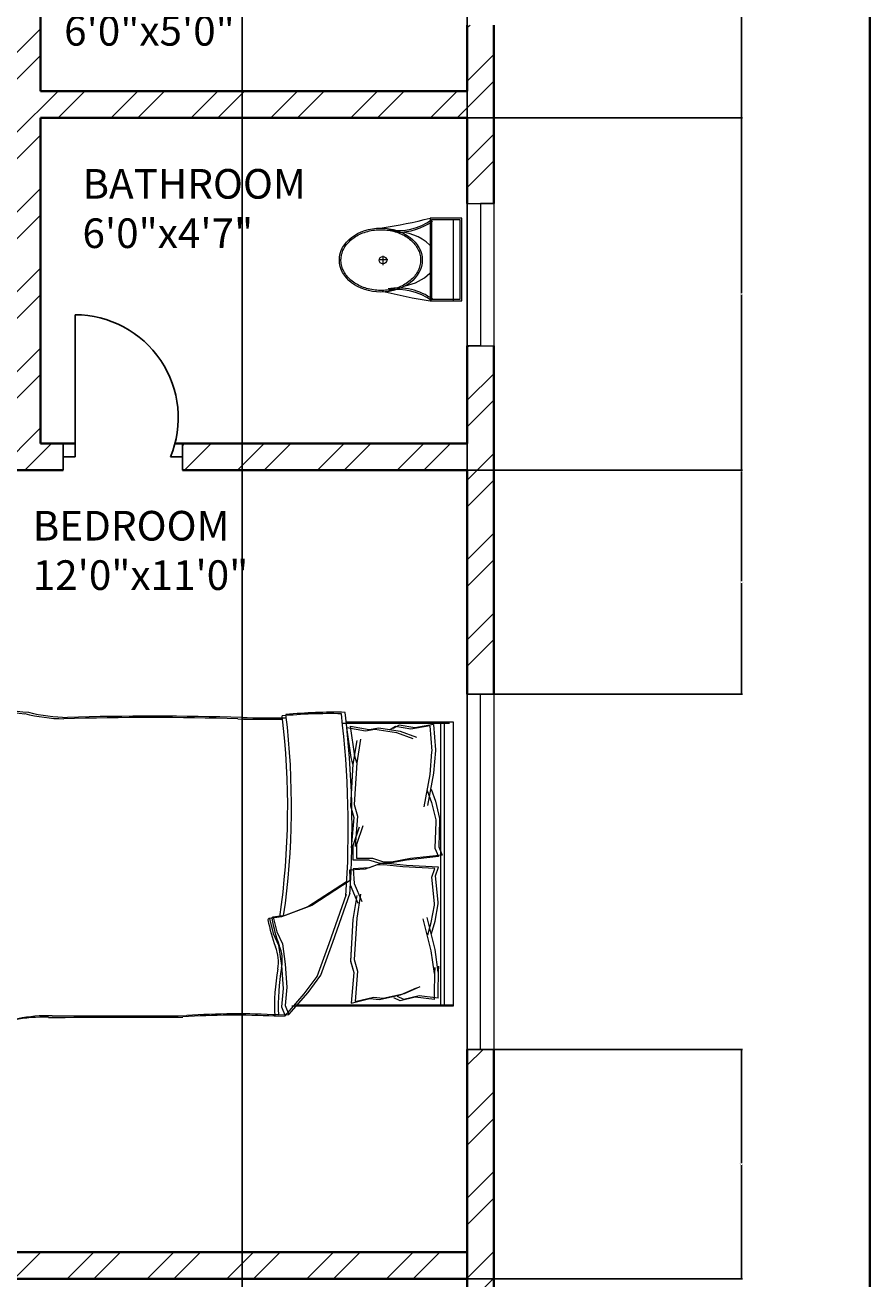
# Model space of a CAD drawing. Units: inches. Extents: x 2063 to 2617, y 1299 to 2210.
# Tile 20 of 22: x 2475 to 2617, y 1727 to 1939. Entities that reach past the tile are written whole.
import ezdxf

# ---------------------------------------------------------------- set-up
doc = ezdxf.new("R2010")
doc.units = ezdxf.units.IN
for name, color, linetype, lineweight in [('A-ANNO-DIMS', 2, 'Continuous', 18), ('A-ANNO-TTLB', 7, 'Continuous', 35), ('A-AREA-IDEN', 7, 'Continuous', 18), ('A-DOOR', 11, 'Continuous', 25), ('A-FLOR-FIXT', 8, 'Continuous', 18), ('A-FURN', 8, 'Continuous', 18), ('A-GLAZ', 123, 'Continuous', 18), ('A-WALL', 7, 'Continuous', 40)]:
    doc.layers.add(name, color=color, linetype=linetype, lineweight=lineweight)
doc.layers.add('A-WALL-PATT', color=215, linetype='Continuous', lineweight=13, true_color=0xa953a0)
doc.styles.get("Standard").update_dxf_attribs({"font": 'arial.ttf'})
doc.dimstyles.get("Standard").update_dxf_attribs({"dimtxt": 0.18, "dimasz": 0.18, "dimexe": 0.18, "dimexo": 0.0625, "dimgap": 0.09, "dimtad": 0, "dimtih": 1, "dimtoh": 1, "dimdec": 4, "dimzin": 0, "dimdsep": 46, "dimtxsty": 'Standard', "dimcen": 0.09, "dimadec": 0, "dimazin": 0, "dimtfac": 1, "dimtdec": 4, "dimtofl": 0, "dimtmove": 0, "dimatfit": 3, "dimfxl": 1, "dimtolj": 1, "dimtzin": 0, "dimarcsym": 0})

# ---------------------------------------------------------------- blocks, each defined once
blk = doc.blocks.new('A$C31115884')
for p, q in [((283.1, 497.7), (223.4, 497.7)), ((257.5, 466.4), (257.5, 523.2)), ((0, 200), (0, 0)), ((520, 200), (0, 200)), ((10, 190), (10, 10)), ((510, 190), (10, 190)), ((510, 10), (510, 190)), ((520, 0), (520, 200)), ((510, 54.5), (0, 54.5)), ((10, 10), (510, 10)), ((0, 0), (520, 0))]:
    blk.add_line(p, q)
blk.add_circle((255.6, 496.4), 23.6)
for centre, radius, start, end in [((2777.7, -204.6), 2807, 165.4549, 171.71327), ((3237, 905), 2807, 188.28673, 194.5451), ((-294.5, 403.3), 364.7, 324.20913, 9.34987), ((-294.5, 403.3), 374.7, 324.20913, 9.34987), ((139.5, 406.2), 293.5, 315.84364, 2.65635), ((805.8, 403.3), 374.7, 179.20365, 215.79087), ((805.8, 403.3), 364.7, 170.65013, 215.79087), ((383.6, 406.2), 293.5, 190.27735, 224.15636)]:
    blk.add_arc(centre, radius, start, end)
blk.add_ellipse((256.2, 509.9), major_axis=(0, -260.7), ratio=0.772727)
blk.add_open_spline([(256.2, 259.2), (263.1, 259.2), (270, 259.7), (287.8, 262.3), (298.7, 265.1), (319.9, 273.1), (330.2, 278.4), (350.1, 291.1), (359.7, 298.7), (377.7, 315.9), (386.2, 325.5), (401.7, 346.6), (408.8, 358.1), (421.3, 382.5), (426.8, 395.5), (435.9, 422.4), (439.5, 436.4), (444.8, 465.1), (446.5, 479.7), (447.9, 509.2), (447.6, 524), (445, 553.3), (442.7, 567.8), (436.3, 596), (432.1, 609.7), (421.9, 636), (416, 648.6), (402.5, 672.1), (395, 683), (378.6, 703), (369.8, 712.1), (351.1, 728), (341.3, 734.8), (320.9, 746.2), (310.4, 750.7), (288.9, 757.3), (278, 759.4), (256, 761), (245, 760.6), (223.1, 757.2), (212.3, 754.3), (191.1, 746.1), (180.8, 740.7), (160.9, 727.8), (151.4, 720.1), (133.5, 702.7), (125.1, 693), (109.6, 671.7), (102.6, 660.2), (90.2, 635.7), (84.9, 622.7), (76, 595.6), (72.4, 581.6), (67.2, 552.9), (65.6, 538.2), (64.4, 508.8), (64.8, 494), (67.5, 464.7), (69.9, 450.2), (76.6, 422), (80.8, 408.3), (91.1, 382.2), (97.2, 369.7), (110.8, 346.3), (118.4, 335.4), (134.8, 315.6), (143.7, 306.7), (162.4, 290.9), (172.3, 284.2), (192.8, 273), (203.3, 268.6), (224.8, 262.2), (235.8, 260.2), (249.9, 259.3), (253, 259.2), (256.2, 259.2)], degree=3, knots=[0, 0, 0, 0, 0.110105, 0.110105, 0.285049, 0.285049, 0.459994, 0.459994, 0.634938, 0.634938, 0.809882, 0.809882, 0.984827, 0.984827, 1.159771, 1.159771, 1.334715, 1.334715, 1.50966, 1.50966, 1.684604, 1.684604, 1.859549, 1.859549, 2.034493, 2.034493, 2.209437, 2.209437, 2.384382, 2.384382, 2.559326, 2.559326, 2.73427, 2.73427, 2.909215, 2.909215, 3.084159, 3.084159, 3.259103, 3.259103, 3.434048, 3.434048, 3.608992, 3.608992, 3.783936, 3.783936, 3.958881, 3.958881, 4.133825, 4.133825, 4.30877, 4.30877, 4.483714, 4.483714, 4.658658, 4.658658, 4.833603, 4.833603, 5.008547, 5.008547, 5.183491, 5.183491, 5.358436, 5.358436, 5.53338, 5.53338, 5.708324, 5.708324, 5.883269, 5.883269, 6.058213, 6.058213, 6.233158, 6.233158, 6.283185, 6.283185, 6.283185, 6.283185])
blk = doc.blocks.new('BED-DOUBLE')
for p, q in [((3.48, 63.33), (3.48, 81.44)), ((3.48, 63.33), (3.48, 81.44)), ((3.48, 81.44), (51.49, 81.44)), ((3.7, 62.69), (3.7, 80.8)), ((3.7, 62.69), (3.7, 80.8)), ((51.27, 81.44), (51.27, 54.83)), ((51.27, 81.44), (51.27, 54.83)), ((51.49, 81.44), (51.49, 80.8)), ((51.49, 80.8), (51.49, 54.19)), ((51.49, 80.8), (51.49, 54.19)), ((3.48, 79.91), (51.27, 79.91)), ((3.48, 79.91), (51.27, 79.91)), ((3.7, 79.27), (51.49, 79.27)), ((3.7, 79.27), (51.49, 79.27)), ((3.9, 78.11), (8.18, 78.43)), ((3.9, 78.11), (8.18, 78.43)), ((8.18, 78.43), (8.29, 78.42)), ((8.18, 78.43), (8.29, 78.42)), ((8.29, 78.42), (12.11, 78.13)), ((8.29, 78.42), (12.11, 78.13)), ((14.86, 77.69), (16.88, 78.42)), ((14.86, 77.69), (16.88, 78.42)), ((16.88, 78.42), (19.77, 79.14)), ((16.88, 78.42), (19.77, 79.14)), ((17.11, 77.78), (20, 78.5)), ((17.11, 77.78), (20, 78.5)), ((19.77, 79.14), (20.09, 79.14)), ((19.77, 79.14), (20.09, 79.14)), ((20, 78.5), (20.32, 78.5)), ((20, 78.5), (20.32, 78.5)), ((20.09, 79.14), (24.54, 79)), ((20.09, 79.14), (24.54, 79)), ((20.32, 78.5), (24.77, 78.36)), ((20.32, 78.5), (24.77, 78.36)), ((24.54, 79), (25.98, 79.57)), ((24.54, 79), (25.98, 79.57)), ((24.77, 78.36), (26.21, 78.93)), ((24.77, 78.36), (26.21, 78.93)), ((25.98, 79.57), (26.56, 74.22)), ((25.98, 79.57), (26.56, 74.22)), ((26.21, 78.93), (26.79, 73.58)), ((26.21, 78.93), (26.79, 73.58)), ((27.98, 78.95), (27.73, 73.58)), ((27.98, 78.95), (27.73, 73.58)), ((29.46, 78.46), (27.98, 78.95)), ((29.46, 78.46), (27.98, 78.95)), ((33.88, 78.89), (29.46, 78.46)), ((33.88, 78.89), (29.46, 78.46)), ((34.21, 78.91), (33.88, 78.89)), ((34.2, 78.91), (33.88, 78.89)), ((37.14, 78.37), (34.2, 78.91)), ((37.14, 78.37), (34.21, 78.91)), ((41.91, 78.37), (36.5, 77.02)), ((41.91, 78.37), (36.5, 77.02)), ((39.2, 77.77), (37.14, 78.37)), ((39.2, 77.77), (37.14, 78.37)), ((45.71, 78.9), (41.91, 78.37)), ((45.71, 78.9), (41.91, 78.37)), ((50.11, 78.89), (44.71, 78.98)), ((44.71, 78.98), (45.71, 78.9)), ((50.11, 78.89), (44.71, 78.98)), ((44.71, 78.98), (45.71, 78.9)), ((50.34, 78.25), (44.94, 78.34)), ((44.94, 78.34), (45.94, 78.26)), ((50.34, 78.25), (44.94, 78.34)), ((44.94, 78.34), (45.94, 78.26)), ((50.11, 78.89), (49.73, 75.68)), ((50.11, 78.89), (49.73, 75.68)), ((3.89, 78.13), (4.47, 74.95)), ((3.9, 78.13), (4.47, 74.95)), ((4.12, 77.49), (4.7, 74.31)), ((4.12, 77.49), (4.7, 74.31)), ((4.13, 77.47), (8.41, 77.8)), ((4.13, 77.47), (8.41, 77.8)), ((8.41, 77.8), (8.51, 77.78)), ((8.41, 77.8), (8.51, 77.78)), ((8.51, 77.78), (12.34, 77.49)), ((8.51, 77.78), (12.34, 77.49)), ((12.11, 78.13), (17.6, 77.12)), ((12.11, 78.13), (17.6, 77.12)), ((12.34, 77.49), (17.83, 76.48)), ((12.34, 77.49), (17.83, 76.48)), ((15.08, 77.05), (17.11, 77.78)), ((15.08, 77.05), (17.11, 77.78)), ((28.21, 78.31), (27.96, 72.94)), ((28.21, 78.31), (27.96, 72.94)), ((29.68, 77.83), (28.21, 78.31)), ((29.68, 77.83), (28.21, 78.31)), ((34.11, 78.25), (29.68, 77.83)), ((34.11, 78.25), (29.68, 77.83)), ((34.43, 78.27), (34.11, 78.25)), ((34.43, 78.27), (34.11, 78.25)), ((37.36, 77.73), (34.43, 78.27)), ((37.36, 77.73), (34.43, 78.27)), ((42.14, 77.73), (36.72, 76.38)), ((42.14, 77.73), (36.72, 76.38)), ((39.43, 77.13), (37.36, 77.73)), ((39.43, 77.13), (37.36, 77.73)), ((45.94, 78.26), (42.14, 77.73)), ((45.94, 78.26), (42.14, 77.73)), ((50.34, 78.25), (49.96, 75.04)), ((50.34, 78.25), (49.96, 75.04)), ((4.47, 74.95), (4.04, 72.34)), ((4.47, 74.95), (4.04, 72.34)), ((4.7, 74.31), (4.27, 71.7)), ((4.7, 74.31), (4.27, 71.7)), ((5.05, 72.49), (6.06, 75.24)), ((5.05, 72.49), (6.06, 75.24)), ((5.28, 71.85), (6.29, 74.6)), ((5.28, 71.85), (6.29, 74.6)), ((26.56, 74.22), (27.14, 71.04)), ((26.56, 74.22), (27.14, 71.04)), ((49.31, 73.19), (48.13, 75.87)), ((49.31, 73.19), (48.13, 75.87)), ((49.54, 72.55), (48.36, 75.23)), ((49.54, 72.55), (48.36, 75.23)), ((49.73, 75.68), (50.33, 73.11)), ((49.73, 75.68), (50.33, 73.11)), ((49.96, 75.04), (50.56, 72.47)), ((49.96, 75.04), (50.56, 72.47)), ((4.04, 72.34), (4.62, 71.33)), ((4.04, 72.34), (4.62, 71.33)), ((4.47, 68.87), (5.05, 72.49)), ((4.47, 68.87), (5.05, 72.49)), ((26.79, 73.58), (27.37, 70.4)), ((26.79, 73.58), (27.37, 70.4)), ((27.73, 73.58), (27.36, 70.37)), ((27.73, 73.58), (27.36, 70.37)), ((27.96, 72.94), (27.58, 69.73)), ((27.96, 72.94), (27.58, 69.73)), ((50.11, 69.61), (49.31, 73.19)), ((50.11, 69.61), (49.31, 73.19)), ((50.34, 68.98), (49.54, 72.55)), ((50.34, 68.98), (49.54, 72.55)), ((50.33, 73.11), (49.81, 72.06)), ((50.33, 73.11), (49.82, 72.06)), ((50.56, 72.47), (50.04, 71.42)), ((50.56, 72.47), (50.04, 71.42)), ((4.27, 71.7), (4.85, 70.69)), ((4.27, 71.7), (4.85, 70.69)), ((4.7, 68.23), (5.28, 71.85)), ((4.7, 68.23), (5.28, 71.85)), ((27.14, 71.04), (27.14, 69.74)), ((27.14, 71.04), (27.14, 69.74)), ((27.36, 70.37), (27.44, 69.07)), ((27.36, 70.37), (27.44, 69.07)), ((27.37, 70.4), (27.37, 69.1)), ((27.37, 70.4), (27.37, 69.1)), ((4.76, 67.28), (4.47, 68.87)), ((4.76, 67.28), (4.47, 68.87)), ((4.99, 66.64), (4.7, 68.23)), ((4.99, 66.64), (4.7, 68.23)), ((27.14, 69.74), (26.56, 67.86)), ((27.14, 69.74), (26.56, 67.86)), ((26.56, 67.86), (26.56, 65.18)), ((26.56, 67.86), (26.56, 65.18)), ((27.37, 69.1), (26.79, 67.22)), ((27.37, 69.1), (26.79, 67.22)), ((27.44, 69.07), (28.13, 67.23)), ((27.44, 69.07), (28.13, 67.23)), ((27.58, 69.73), (27.66, 68.43)), ((27.58, 69.73), (27.66, 68.43)), ((27.66, 68.43), (28.36, 66.59)), ((27.66, 68.43), (28.36, 66.59)), ((49.92, 68.01), (50.11, 69.61)), ((49.92, 68.01), (50.11, 69.61)), ((50.7, 64.87), (49.92, 68.01)), ((50.7, 64.87), (49.92, 68.01)), ((50.15, 67.37), (50.34, 68.98)), ((50.15, 67.37), (50.34, 68.98)), ((4.18, 64.1), (4.76, 67.28)), ((4.18, 64.1), (4.76, 67.28)), ((4.41, 63.46), (4.99, 66.64)), ((4.41, 63.46), (4.99, 66.64)), ((6.38, 65.82), (10.41, 65.15)), ((6.38, 65.82), (10.41, 65.15)), ((24.1, 65.18), (20.96, 66.27)), ((24.1, 65.18), (20.96, 66.27)), ((24.33, 64.54), (21.19, 65.63)), ((24.33, 64.54), (21.19, 65.63)), ((26.79, 67.22), (26.79, 64.54)), ((26.79, 67.22), (26.79, 64.54)), ((28.13, 67.23), (28.3, 64.55)), ((28.13, 67.23), (28.3, 64.55)), ((28.36, 66.59), (28.53, 63.91)), ((28.36, 66.59), (28.53, 63.91)), ((30.75, 64.7), (33.82, 65.99)), ((30.75, 64.7), (33.82, 65.99)), ((32.56, 65.82), (36.6, 65.15)), ((32.56, 65.82), (36.6, 65.15)), ((50.93, 64.23), (50.15, 67.37)), ((50.93, 64.23), (50.15, 67.37)), ((9.28, 64.83), (4.18, 64.1)), ((9.28, 64.83), (4.18, 64.1)), ((9.51, 64.19), (4.41, 63.46)), ((9.51, 64.19), (4.41, 63.46)), ((6.61, 65.18), (10.64, 64.51)), ((6.61, 65.18), (10.64, 64.51)), ((10.41, 65.15), (9.28, 64.83)), ((10.41, 65.15), (9.28, 64.83)), ((10.64, 64.51), (9.51, 64.19)), ((10.64, 64.51), (9.51, 64.19)), ((10.41, 65.15), (17.42, 64.72)), ((10.41, 65.15), (17.42, 64.72)), ((10.64, 64.51), (17.65, 64.08)), ((10.64, 64.51), (17.65, 64.08)), ((17.42, 64.72), (19.38, 65.27)), ((17.42, 64.72), (19.38, 65.27)), ((17.65, 64.08), (19.61, 64.64)), ((17.65, 64.08), (19.61, 64.64)), ((19.38, 65.27), (24.52, 64.87)), ((19.38, 65.27), (24.52, 64.87)), ((19.61, 64.64), (24.74, 64.23)), ((19.61, 64.64), (24.74, 64.23)), ((26.56, 65.18), (24.1, 65.18)), ((26.56, 65.18), (24.1, 65.18)), ((26.79, 64.54), (24.33, 64.54)), ((26.79, 64.54), (24.33, 64.54)), ((28.3, 64.55), (30.75, 64.7)), ((28.3, 64.55), (30.75, 64.7)), ((28.53, 63.91), (30.98, 64.06)), ((28.53, 63.91), (30.98, 64.06)), ((30.26, 64.06), (34.45, 57.57)), ((30.26, 64.06), (34.45, 57.57)), ((30.98, 64.06), (34.05, 65.35)), ((30.98, 64.06), (34.05, 65.35)), ((40.64, 61.13), (32.31, 64.06)), ((40.64, 61.13), (32.31, 64.06)), ((32.79, 65.18), (36.83, 64.51)), ((32.79, 65.18), (36.82, 64.51)), ((36.6, 65.15), (43.61, 64.72)), ((36.6, 65.15), (43.61, 64.72)), ((36.82, 64.51), (43.83, 64.08)), ((36.83, 64.51), (43.84, 64.08)), ((43.61, 64.72), (45.57, 65.27)), ((43.61, 64.72), (45.57, 65.27)), ((43.83, 64.08), (45.8, 64.64)), ((43.84, 64.08), (45.8, 64.64)), ((45.57, 65.27), (50.7, 64.87)), ((45.57, 65.27), (50.7, 64.87)), ((45.8, 64.64), (50.93, 64.23)), ((45.8, 64.64), (50.93, 64.23)), ((30.49, 63.42), (34.68, 56.93)), ((30.49, 63.42), (34.68, 56.93)), ((40.87, 60.49), (32.53, 63.42)), ((40.87, 60.49), (32.54, 63.42)), ((46.22, 59.11), (40.64, 61.13)), ((46.22, 59.11), (40.64, 61.13)), ((46.45, 58.48), (40.87, 60.49)), ((46.45, 58.48), (40.87, 60.49)), ((34.45, 57.57), (36.15, 53.08)), ((34.45, 57.57), (36.15, 53.08)), ((49.16, 56.95), (46.22, 59.11)), ((49.16, 56.95), (46.22, 59.11)), ((49.39, 56.31), (46.45, 58.48)), ((49.39, 56.31), (46.45, 58.48)), ((34.68, 56.93), (36.38, 52.44)), ((34.68, 56.93), (36.38, 52.44)), ((52.87, 53.7), (49.16, 56.95)), ((52.87, 53.7), (49.16, 56.95)), ((53.1, 53.06), (49.39, 56.31)), ((53.1, 53.06), (49.39, 56.31)), ((36.15, 53.08), (36.46, 51.07)), ((36.15, 53.08), (36.46, 51.07)), ((40.95, 52.61), (44.36, 53.08)), ((40.95, 52.61), (44.36, 53.08)), ((44.36, 53.08), (48.23, 53.39)), ((44.36, 53.08), (48.23, 53.39)), ((48.23, 53.39), (51.33, 53.08)), ((48.23, 53.39), (51.33, 53.08)), ((51.33, 53.08), (52.87, 53.7)), ((51.33, 53.08), (52.87, 53.7)), ((51.56, 52.44), (53.1, 53.06)), ((51.56, 52.44), (53.1, 53.06)), ((52.95, 51.95), (52.87, 53.7, 3.87)), ((52.95, 51.95), (52.87, 53.7, 3.87)), ((53.18, 51.31), (53.1, 53.06, 3.87)), ((53.18, 51.31), (53.1, 53.06, 3.87)), ((36.38, 52.44), (36.69, 50.43)), ((36.38, 52.44), (36.69, 50.43)), ((36.46, 51.07), (38.94, 51.69)), ((36.46, 51.07), (38.94, 51.69)), ((36.69, 50.43), (39.17, 51.05)), ((36.69, 50.43), (39.17, 51.05)), ((38.94, 51.69), (40.95, 52.61)), ((38.94, 51.69), (40.95, 52.61)), ((39.17, 51.05), (41.18, 51.97)), ((39.17, 51.05), (41.18, 51.97)), ((41.18, 51.97), (44.59, 52.44)), ((41.18, 51.97), (44.59, 52.44)), ((44.59, 52.44), (48.46, 52.75)), ((44.59, 52.44), (48.46, 52.75)), ((48.46, 52.75), (51.56, 52.44)), ((48.46, 52.75), (51.56, 52.44)), ((15.06, 2.2), (39.68, 2.2)), ((15.06, 2.2), (39.68, 2.2)), ((15.29, 1.56), (39.91, 1.56)), ((15.29, 1.56), (39.91, 1.56))]:
    blk.add_line(p, q)
for centre, radius, start, end in [((21.36, -100.61), 164.97, 86.0865, 96.7821), ((21.36, -100.61), 164.97, 86.0865, 96.7821), ((21.59, -101.25), 164.97, 86.0865, 96.7821), ((21.59, -101.25), 164.97, 86.0865, 96.7821), ((85.16, 61.35), 83.31, 178.7218, 185.604), ((85.16, 61.35), 83.31, 178.7218, 185.604), ((85.39, 60.71), 83.31, 178.7218, 185.604), ((85.39, 60.71), 83.31, 178.7218, 185.604), ((17.76, -74.87), 129.02, 81.7845, 96.9006), ((17.76, -74.87), 129.02, 81.7845, 96.9006), ((17.98, -75.51), 129.02, 81.7845, 96.9006), ((17.98, -75.51), 129.02, 81.7845, 96.9006), ((-167.31, 50.27), 170.11, 358.4762, 1.0082), ((-167.31, 50.27), 170.11, 358.4762, 1.0082), ((-167.08, 49.63), 170.11, 358.4762, 1.0082), ((-167.08, 49.63), 170.11, 358.4762, 1.0082), ((36.64, 51), 0.185, 160.2464, 271.1377), ((36.64, 51), 0.185, 160.2464, 271.1377), ((31.15, 79.96), 29.65, 280.6617, 289.8806), ((31.15, 79.96), 29.65, 280.6617, 289.8806), ((31.38, 79.32), 29.65, 280.6617, 289.8806), ((31.38, 79.32), 29.65, 280.6617, 289.8806), ((43.74, 46.38), 6.22, 78.6608, 113.7384), ((43.74, 46.38), 6.22, 78.6608, 113.7384), ((43.97, 45.74), 6.22, 78.6608, 113.7384), ((43.97, 45.74), 6.22, 78.6608, 113.7384), ((51.33, 88.1), 36.18, 259.8763, 272.5657), ((51.33, 88.1), 36.18, 259.8763, 272.5657), ((51.56, 87.46), 36.18, 259.8763, 272.5657), ((51.56, 87.46), 36.18, 259.8763, 272.5657), ((182.27, 45.13), 129.5, 176.9791, 183.8365), ((182.27, 45.13), 129.5, 176.9791, 183.8365), ((182.49, 44.49), 129.5, 176.9791, 183.8365), ((182.49, 44.49), 129.5, 176.9791, 183.8365), ((36.87, 50.36), 0.185, 160.2464, 271.1377), ((36.86, 50.36), 0.185, 160.2464, 271.1377), ((484.82, 30.83), 482.31, 178.2277, 181.7185), ((484.82, 30.83), 482.31, 178.2277, 181.7185), ((485.05, 30.19), 482.31, 178.2277, 181.7185), ((485.05, 30.19), 482.31, 178.2277, 181.7185), ((-4508.74, 13.62), 4561.86, 0.00217, 0.28689), ((-4508.74, 13.62), 4561.86, 0.00217, 0.28689), ((-4508.51, 12.98), 4561.86, 0.00217, 0.28689), ((-4508.51, 12.98), 4561.86, 0.00217, 0.28689), ((-26.9, 16.93), 29.63, 346.0648, 358.9113), ((-26.9, 16.93), 29.63, 346.0648, 358.9113), ((-26.67, 16.29), 29.63, 346.0648, 358.9113), ((-26.67, 16.29), 29.63, 346.0648, 358.9113), ((76.16, 12.78), 23.07, 177.4714, 206.4681), ((76.16, 12.78), 23.07, 177.4714, 206.4681), ((76.39, 12.14), 23.07, 177.4714, 206.4681), ((76.39, 12.14), 23.07, 177.4714, 206.4681), ((-21.66, 11.17), 23.56, 337.9751, 356.652), ((-21.66, 11.17), 23.56, 337.9751, 356.652), ((-21.43, 10.53), 23.56, 337.9751, 356.652), ((-21.43, 10.53), 23.56, 337.9751, 356.652), ((1.09, 1.73), 1.09, 146.1736, 293.4781), ((1.09, 1.73), 1.09, 146.1736, 293.4781), ((21.43, -119.39), 121.76, 92.9958, 99.4091), ((21.43, -119.39), 121.76, 92.9958, 99.4091), ((-17.22, 105.16), 106.46, 283.3832, 287.7053), ((-17.22, 105.16), 106.46, 283.3832, 287.7053), ((-16.99, 104.52), 106.46, 283.3832, 287.7053), ((-16.99, 104.52), 106.46, 283.3832, 287.7053), ((41.15, -130.83), 133.04, 84.4998, 90.6351), ((41.15, -130.83), 133.04, 84.4998, 90.6351), ((54.41, 2.57), 1.1, 242.6588, 356.02), ((54.41, 2.57), 1.1, 242.6588, 356.02), ((1.32, 1.09), 1.09, 146.1736, 293.4781), ((1.32, 1.09), 1.09, 146.1736, 293.4781), ((21.66, -120.03), 121.76, 92.9958, 99.4091), ((21.66, -120.03), 121.76, 92.9958, 99.4091), ((41.38, -131.47), 133.04, 84.4998, 90.6351), ((41.38, -131.47), 133.04, 84.4998, 90.6351), ((54.64, 1.93), 1.1, 242.6588, 356.02), ((54.64, 1.93), 1.1, 242.6588, 356.02)]:
    blk.add_arc(centre, radius, start, end)
blk = doc.blocks.new('WIN-24IN')
for p, q in [((0, 24), (4.5, 24)), ((0, 24), (0, 0)), ((4.5, 24), (2.25, 24)), ((2.25, 24), (2.25, 0)), ((4.5, 24), (4.5, 0)), ((2.25, 0), (0, 0)), ((0, 0), (4.5, 0))]:
    blk.add_line(p, q)
blk = doc.blocks.new('*D43')
at = {"layer": 'A-ANNO-DIMS', "color": 0, "lineweight": -2, "transparency": 16777216}
for p, q in [((2549.21, 1766.03), (2595.57, 1766.03)), ((2595.39, 1765.85), (2595.39, 1746.85)), ((2595.39, 1727.49), (2595.39, 1746.49)), ((2549.21, 1727.31), (2595.57, 1727.31))]:
    blk.add_line(p, q, dxfattribs=at)
at = {"layer": 'A-ANNO-DIMS', "color": 0, "transparency": 16777216}
for points in [[(2595.36, 1765.85), (2595.42, 1765.85), (2595.39, 1766.03)], [(2595.36, 1727.49), (2595.42, 1727.49), (2595.39, 1727.31)]]:
    blk.add_solid(points, dxfattribs=at)
at = {"layer": 'Defpoints', "color": 0, "transparency": 16777216}
for p in [(2549.14, 1766.03), (2595.39, 1766.03), (2549.14, 1727.31)]:
    blk.add_point(p, dxfattribs=at)
at = {"layer": 'A-ANNO-DIMS', "color": 0, "transparency": 16777216, "insert": (2595.39, 1746.67), "char_height": 0.18, "attachment_point": 5}
blk.add_mtext('\\A1;38.72', dxfattribs=at)
blk = doc.blocks.new('*D44')
at = {"layer": 'A-ANNO-DIMS', "color": 0, "lineweight": -2, "transparency": 16777216}
for p, q in [((2549.21, 1863.81), (2595.57, 1863.81)), ((2595.39, 1863.63), (2595.39, 1845.1)), ((2595.39, 1826.21), (2595.39, 1844.74)), ((2549.21, 1826.03), (2595.57, 1826.03))]:
    blk.add_line(p, q, dxfattribs=at)
at = {"layer": 'A-ANNO-DIMS', "color": 0, "transparency": 16777216}
for points in [[(2595.36, 1863.63), (2595.42, 1863.63), (2595.39, 1863.81)], [(2595.36, 1826.21), (2595.42, 1826.21), (2595.39, 1826.03)]]:
    blk.add_solid(points, dxfattribs=at)
at = {"layer": 'Defpoints', "color": 0, "transparency": 16777216}
for p in [(2549.14, 1863.81), (2595.39, 1863.81), (2549.14, 1826.03)]:
    blk.add_point(p, dxfattribs=at)
at = {"layer": 'A-ANNO-DIMS', "color": 0, "transparency": 16777216, "insert": (2595.39, 1844.92), "char_height": 0.18, "attachment_point": 5}
blk.add_mtext('\\A1;37.78', dxfattribs=at)
blk = doc.blocks.new('*D45')
at = {"layer": 'A-ANNO-DIMS', "color": 0, "lineweight": -2, "transparency": 16777216}
for p, q in [((2549.21, 1923.31), (2595.57, 1923.31)), ((2595.39, 1923.13), (2595.39, 1893.74)), ((2595.39, 1863.99), (2595.39, 1893.38)), ((2549.21, 1863.81), (2595.57, 1863.81))]:
    blk.add_line(p, q, dxfattribs=at)
at = {"layer": 'A-ANNO-DIMS', "color": 0, "transparency": 16777216}
for points in [[(2595.36, 1923.13), (2595.42, 1923.13), (2595.39, 1923.31)], [(2595.36, 1863.99), (2595.42, 1863.99), (2595.39, 1863.81)]]:
    blk.add_solid(points, dxfattribs=at)
at = {"layer": 'Defpoints', "color": 0, "transparency": 16777216}
for p in [(2549.14, 1923.31), (2595.39, 1923.31), (2549.14, 1863.81)]:
    blk.add_point(p, dxfattribs=at)
at = {"layer": 'A-ANNO-DIMS', "color": 0, "transparency": 16777216, "insert": (2595.39, 1893.56), "char_height": 0.18, "attachment_point": 5}
blk.add_mtext('\\A1;59.5', dxfattribs=at)
blk = doc.blocks.new('*D46')
at = {"layer": 'A-ANNO-DIMS', "color": 0, "lineweight": -2, "transparency": 16777216}
for p, q in [((2549.21, 1975.81), (2595.57, 1975.81)), ((2595.39, 1975.63), (2595.39, 1949.74)), ((2595.39, 1923.49), (2595.39, 1949.38)), ((2549.21, 1923.31), (2595.57, 1923.31))]:
    blk.add_line(p, q, dxfattribs=at)
at = {"layer": 'A-ANNO-DIMS', "color": 0, "transparency": 16777216}
for points in [[(2595.36, 1975.63), (2595.42, 1975.63), (2595.39, 1975.81)], [(2595.36, 1923.49), (2595.42, 1923.49), (2595.39, 1923.31)]]:
    blk.add_solid(points, dxfattribs=at)
at = {"layer": 'Defpoints', "color": 0, "transparency": 16777216}
for p in [(2549.14, 1975.81), (2595.39, 1975.81), (2549.14, 1923.31)]:
    blk.add_point(p, dxfattribs=at)
at = {"layer": 'A-ANNO-DIMS', "color": 0, "transparency": 16777216, "insert": (2595.39, 1949.56), "char_height": 0.18, "attachment_point": 5}
blk.add_mtext('\\A1;52.5', dxfattribs=at)
blk = doc.blocks.new('*D52')
at = {"layer": 'A-ANNO-DIMS', "color": 0, "lineweight": -2, "transparency": 16777216}
for p, q in [((2511.17, 2124.25), (2511.17, 1317.7)), ((2549.14, 2124.25), (2549.14, 1317.7)), ((2511.35, 1317.88), (2529.69, 1317.88)), ((2548.96, 1317.88), (2530.62, 1317.88))]:
    blk.add_line(p, q, dxfattribs=at)
at = {"layer": 'A-ANNO-DIMS', "color": 0, "transparency": 16777216}
for points in [[(2511.35, 1317.91), (2511.35, 1317.85), (2511.17, 1317.88)], [(2548.96, 1317.91), (2548.96, 1317.85), (2549.14, 1317.88)]]:
    blk.add_solid(points, dxfattribs=at)
at = {"layer": 'Defpoints', "color": 0, "transparency": 16777216}
for p in [(2511.17, 2124.31), (2549.14, 2124.31), (2549.14, 1317.88)]:
    blk.add_point(p, dxfattribs=at)
at = {"layer": 'A-ANNO-DIMS', "color": 0, "transparency": 16777216, "insert": (2530.16, 1317.88), "char_height": 0.18, "attachment_point": 5}
blk.add_mtext('\\A1;37.974', dxfattribs=at)

msp = doc.modelspace()

# ---------------------------------------------------------------- hatches: boundary and pattern name
at = {"layer": 'A-WALL-PATT'}
h = msp.add_hatch(dxfattribs=at)
h.set_pattern_fill('ANSI32', color=256)
h.paths.add_polyline_path([(2553.6442, 2128.8122), (2511.1703, 2128.8122), (2511.1703, 2124.3122), (2549.1442, 2124.3122), (2549.1442, 2095.662), (2553.6442, 2095.662)])
h.paths.add_polyline_path([(2553.6442, 2035.662), (2549.1442, 2035.662), (2549.1442, 1980.3122), (2503.7214, 1980.3122), (2503.7214, 1975.8122), (2549.1442, 1975.8122), (2549.1442, 1962.9693), (2553.6442, 1962.9693)])
h.paths.add_polyline_path([(2553.6442, 1938.9693), (2549.1442, 1938.9693), (2549.1442, 1927.8122), (2477.1442, 1927.8122), (2477.1442, 1975.8122), (2481.2918, 1975.8122), (2481.2918, 1980.3122), (2453.2648, 1980.3122), (2453.2648, 1975.8122), (2472.6442, 1975.8122), (2472.6442, 1868.3122), (2400.6442, 1868.3122), (2400.6442, 1861.3782), (2405.1442, 1861.3782), (2405.1442, 1863.8122), (2480.9699, 1863.8122), (2480.9699, 1866.0622), (2480.9699, 1868.3122), (2477.1442, 1868.3122), (2477.1442, 1923.3122), (2549.1442, 1923.3122), (2549.1442, 1908.8504), (2553.6442, 1908.8504)])
h.paths.add_polyline_path([(2553.6442, 1884.8504), (2549.1442, 1884.8504), (2549.1442, 1868.3122), (2501.0636, 1868.3122), (2501.0636, 1863.8122), (2549.1442, 1863.8122), (2549.1442, 1826.0298), (2553.6442, 1826.0298)])
h.paths.add_polyline_path([(2388.1504, 1980.3122), (2340.6442, 1980.3122), (2340.6442, 2124.3122), (2358.7501, 2124.3122), (2358.7501, 2128.8122), (2316.3482, 2128.8122), (2316.3482, 2124.3122), (2336.1442, 2124.3122), (2336.1442, 1980.3122), (2289.1737, 1980.3122), (2289.1737, 1975.8122), (2336.1442, 1975.8122), (2336.1442, 1619.3122), (2333.1433, 1619.3122), (2333.1433, 1614.8122), (2344.1671, 1614.8122), (2344.1671, 1617.0622), (2344.1671, 1619.3122), (2340.6442, 1619.3122), (2340.6442, 1975.8122), (2388.1504, 1975.8122), (2388.1504, 1978.0622)])
h.paths.add_polyline_path([(2290.1442, 1614.8122), (2301.4594, 1614.8122), (2301.4594, 1617.0622), (2301.4594, 1619.3122), (2285.6442, 1619.3122), (2285.6442, 1566.8122), (2280.8619, 1566.8122), (2280.8619, 1564.5622), (2280.8619, 1562.3122), (2285.6442, 1562.3122), (2285.6442, 1442.3122), (2281.7879, 1442.3122), (2281.7879, 1437.8122), (2285.6442, 1437.8122), (2285.6442, 1401.8122), (2290.1442, 1401.8122)])
h.paths.add_polyline_path([(2549.1442, 1731.8122), (2405.1442, 1731.8122), (2405.1442, 1834.4638), (2402.8942, 1834.4638), (2400.6442, 1834.4638), (2400.6442, 1727.3122), (2549.1442, 1727.3122)])
h.paths.add_polyline_path([(2553.6442, 1766.0298), (2551.3942, 1766.0298), (2549.1442, 1766.0298), (2549.1442, 1686.7767), (2553.6442, 1686.7767)])
h.paths.add_polyline_path([(2553.6442, 1638.7767), (2551.3942, 1638.7767), (2549.1442, 1638.7767), (2549.1442, 1619.3122), (2448.6442, 1619.3122), (2448.6442, 1610.5671), (2450.8942, 1610.5671), (2453.1442, 1610.5671), (2453.1442, 1614.8122), (2549.1442, 1614.8122), (2549.1442, 1601.6421), (2553.6442, 1601.6421)])
h.paths.add_polyline_path([(2553.6442, 1577.6421), (2551.3942, 1577.6421), (2549.1442, 1577.6421), (2549.1442, 1566.8122), (2453.1442, 1566.8122), (2453.1442, 1591.5045), (2451.0335, 1591.5045), (2448.6442, 1591.5045), (2448.6442, 1566.8122), (2434.0475, 1566.8122), (2434.0475, 1562.3122), (2549.1442, 1562.3122), (2549.1442, 1533.48), (2553.6442, 1533.48)])
h.paths.add_polyline_path([(2553.6442, 1473.48), (2549.1442, 1473.48), (2549.1442, 1442.3122), (2502.6258, 1442.3122), (2502.6258, 1437.8122), (2549.1442, 1437.8122), (2549.1442, 1401.8122), (2553.6442, 1401.8122)])
h.paths.add_polyline_path([(2395.6442, 1562.3122), (2400.0901, 1562.3122), (2400.0901, 1564.5622), (2400.0901, 1566.8122), (2395.6442, 1566.8122), (2395.6442, 1619.3122), (2379.1127, 1619.3122), (2379.1127, 1614.8122), (2391.1442, 1614.8122), (2391.1442, 1401.8122), (2395.6442, 1401.8122), (2395.6442, 1437.8122), (2399.2425, 1437.8122), (2399.2425, 1440.0622), (2399.2425, 1442.3122), (2395.6442, 1442.3122)])
h.paths.add_polyline_path([(2442.6258, 1442.3122), (2419.6262, 1442.3122), (2419.6262, 1437.8122), (2442.6258, 1437.8122), (2442.6258, 1440.0622)])
h.paths.add_polyline_path([(2127.6442, 1480.2532), (2125.3942, 1480.2532), (2123.1442, 1480.2532), (2123.1442, 1401.8122), (2127.6442, 1401.8122), (2127.6442, 1437.8122), (2145.1538, 1437.8122), (2145.1538, 1440.0622), (2145.1538, 1442.3122), (2127.6442, 1442.3122)])
h.paths.add_polyline_path([(2259.809, 1442.3122), (2205.1538, 1442.3122), (2205.1538, 1437.8122), (2259.809, 1437.8122), (2259.809, 1440.0622)])
h.paths.add_polyline_path([(2127.6442, 1659.7652), (2123.1442, 1659.7652), (2123.1442, 1605.5161), (2125.3942, 1605.5161), (2127.6442, 1605.5161), (2127.6442, 1614.8122), (2223.6442, 1614.8122), (2223.6442, 1611.2723), (2228.1442, 1611.2723), (2228.1442, 1619.3122), (2127.6442, 1619.3122)])
h.paths.add_polyline_path([(2244.8673, 1566.8122), (2228.1442, 1566.8122), (2228.1442, 1590.8122), (2225.8942, 1590.8122), (2223.6442, 1590.8122), (2223.6442, 1566.8122), (2127.6442, 1566.8122), (2127.6442, 1581.5161), (2123.1442, 1581.5161), (2123.1442, 1540.2532), (2127.6442, 1540.2532), (2127.6442, 1562.3122), (2244.8673, 1562.3122), (2244.8673, 1564.5622)])
h.paths.add_polyline_path([(2172.5174, 1868.3122), (2127.6442, 1868.3122), (2127.6442, 1886.5833), (2123.1442, 1886.5833), (2123.1442, 1832.6633), (2127.6442, 1832.6633), (2127.6442, 1863.8122), (2172.5174, 1863.8122), (2172.5174, 1866.0622)])
h.paths.add_polyline_path([(2276.1442, 1868.3122), (2204.1442, 1868.3122), (2204.1442, 1923.3122), (2204.1442, 1975.8122), (2224.8362, 1975.8122), (2224.8362, 1978.1097), (2224.8362, 1980.3122), (2195.0729, 1980.3122), (2195.0729, 1978.0622), (2195.0729, 1975.8122), (2199.6442, 1975.8122), (2199.6442, 1927.8122), (2127.6442, 1927.8122), (2127.6442, 1942.3492), (2123.1442, 1942.3492), (2123.1442, 1910.5833), (2127.6442, 1910.5833), (2127.6442, 1923.3122), (2199.6442, 1923.3122), (2199.6442, 1868.3122), (2194.8228, 1868.3122), (2194.8228, 1864.7337), (2194.8228, 1863.8122), (2271.6442, 1863.8122), (2271.6442, 1860.0507), (2276.1442, 1860.0507)])
h.paths.add_polyline_path([(2276.1442, 1829.994), (2273.8942, 1829.994), (2271.6442, 1829.994), (2271.6442, 1731.8122), (2127.6442, 1731.8122), (2127.6442, 1772.6633), (2123.1442, 1772.6633), (2123.1442, 1707.7652), (2127.6442, 1707.7652), (2127.6442, 1727.3122), (2276.1442, 1727.3122)])
h.paths.add_polyline_path([(2127.6442, 2022.1152), (2123.1442, 2022.1152), (2123.1442, 1966.3492), (2127.6442, 1966.3492), (2127.6442, 1975.8122), (2174.2082, 1975.8122), (2174.2082, 1978.0622), (2174.2082, 1980.3122), (2127.6442, 1980.3122)])
h.paths.add_polyline_path([(2361.9755, 1678.588), (2398.4558, 1678.588), (2398.4558, 1697.2453), (2361.9755, 1697.2453)], flags=9)
h.paths.add_polyline_path([(2351.5397, 1780.4072), (2386.1987, 1780.4072), (2386.1987, 1790.7107), (2351.5397, 1790.7107)], flags=25)
h.paths.add_polyline_path([(2350.6753, 1940.9321), (2387.6024, 1940.9321), (2387.6024, 1959.5894), (2350.6753, 1959.5894)], flags=25)
h.paths.add_polyline_path([(2254.9545, 1684.638), (2295.0943, 1684.638), (2295.0943, 1703.2953), (2254.9545, 1703.2953)], flags=9)
h.paths.add_polyline_path([(2282.4946, 1782.4438), (2317.1535, 1782.4438), (2317.1535, 1792.7474), (2282.4946, 1792.7474)], flags=9)
h.paths.add_polyline_path([(2270.327, 1939.2854), (2307.254, 1939.2854), (2307.254, 1957.9428), (2270.327, 1957.9428)], flags=9)

# ---------------------------------------------------------------- linework, layer by layer
at = {"layer": 'A-ANNO-TTLB'}
msp.add_lwpolyline([(2062.5792, 2209.6485), (2617.0648, 2209.6485), (2617.0648, 1299.1125), (2062.5792, 1299.1125)], close=True, dxfattribs=at)
at = {"layer": 'A-DOOR'}
for p, q in [((2482.9699, 1866.0622), (2482.9699, 1890.0622)), ((2480.9699, 1868.3122), (2480.9699, 1863.8122)), ((2501.0636, 1868.3122), (2501.0636, 1863.8122)), ((2480.9699, 1863.8122), (2480.9699, 1866.0622)), ((2480.9699, 1866.0622), (2482.9699, 1866.0622)), ((2501.0636, 1866.0622), (2499.0636, 1866.0622)), ((2501.0636, 1863.8122), (2501.0636, 1866.0622))]:
    msp.add_line(p, q, dxfattribs=at)
msp.add_arc((2482.9699, 1872.6662), 17.396, 337.689352, 90, dxfattribs=at)
at = {"layer": 'A-GLAZ'}
for p, q in [((2551.3942, 1826.0298), (2549.1442, 1826.0298)), ((2549.1442, 1826.0298), (2553.6442, 1826.0298)), ((2549.1442, 1826.0298), (2549.1442, 1764.1588)), ((2551.3942, 1766.0298), (2551.3942, 1826.0298)), ((2553.6442, 1826.0298), (2553.6442, 1766.0298)), ((2549.1442, 1766.0298), (2553.6442, 1766.0298)), ((2553.6442, 1766.0298), (2551.3942, 1766.0298))]:
    msp.add_line(p, q, dxfattribs=at)
at = {"layer": 'A-WALL'}
for p, q in [((2477.1442, 1975.8122), (2477.1442, 1927.8122)), ((2549.1442, 1938.9693), (2549.1442, 1927.8122)), ((2553.6442, 1938.9693), (2553.6442, 1908.8504)), ((2477.1442, 1927.8122), (2549.1442, 1927.8122)), ((2477.1442, 1923.3122), (2549.1442, 1923.3122)), ((2477.1442, 1923.3122), (2477.1442, 1868.3122)), ((2549.1442, 1923.3122), (2549.1442, 1908.8504)), ((2549.1442, 1884.8504), (2549.1442, 1868.3122)), ((2553.6442, 1884.8504), (2553.6442, 1826.0298)), ((2477.1442, 1868.3122), (2482.9699, 1868.3122)), ((2499.8122, 1868.3122), (2549.1442, 1868.3122)), ((2405.1442, 1863.8122), (2480.9699, 1863.8122)), ((2501.0636, 1863.8122), (2549.1442, 1863.8122)), ((2549.1442, 1863.8122), (2549.1442, 1826.0298)), ((2549.1442, 1766.0298), (2549.1442, 1686.7767)), ((2553.6442, 1766.0298), (2553.6442, 1686.7767)), ((2405.1442, 1731.8122), (2549.1442, 1731.8122)), ((2400.6442, 1727.3122), (2549.1442, 1727.3122))]:
    msp.add_line(p, q, dxfattribs=at)

# ---------------------------------------------------------------- block references
at = {"layer": 'A-FLOR-FIXT', "xscale": 0.0268011493576733, "yscale": 0.0268011493576733, "zscale": 0.0268011493576733, "rotation": 89.99999999999999}
msp.add_blockref('A$C31115884', (2548.213, 1892.4371), dxfattribs=at)
at = {"layer": 'A-FURN', "rotation": 270}
msp.add_blockref('BED-DOUBLE', (2465.3294, 1824.819), dxfattribs=at)
at = {"layer": 'A-GLAZ'}
msp.add_blockref('WIN-24IN', (2549.144, 1884.8501), dxfattribs=at)

# ---------------------------------------------------------------- texts
at = {"layer": 'A-AREA-IDEN', "char_height": 5, "attachment_point": 1}
for s, width, insert in [('BATHROOM\\P6\'0"x5\'0"', 102.054079, (2481.1209, 1948.8348)), ('BATHROOM\\P6\'0"x4\'7"', 176.148075, (2484.2186, 1914.67)), ('BEDROOM\\P12\'0"x11\'0"', 143.003661, (2475.8257, 1856.9541))]:
    msp.add_mtext_dynamic_manual_height_columns(s, width=width, gutter_width=12.5, heights=[0], dxfattribs=dict(at, insert=insert))

# ---------------------------------------------------------------- dimensions: what is measured, and where the dimension line sits
at = {"layer": 'A-ANNO-DIMS'}
dim = msp.add_linear_dim(base=(2549.1442, 1317.8821), p1=(2511.1703, 2124.3122), p2=(2549.1442, 2124.3122), dimstyle='Standard', override={"dimdec": 3, "dimlfac": 1, "dimrnd": 0, "dimzin": 0, "dimdsep": 46, "dimlunit": 2}, dxfattribs=at)
dim.commit()
dim.dimension.update_dxf_attribs({"geometry": '*D52', "text_midpoint": (2530.1573, 1317.8821)})
for base, p1, p2, override, picture, middle in [((2595.3943, 1975.8122), (2549.1442, 1923.3122), (2549.1442, 1975.8122), {"dimdec": 1, "dimlfac": 1, "dimrnd": 0, "dimzin": 0, "dimdsep": 46, "dimlunit": 2}, '*D46', (2595.3943, 1949.5622)), ((2595.3943, 1923.3122), (2549.1442, 1863.8122), (2549.1442, 1923.3122), {"dimdec": 1, "dimlfac": 1, "dimrnd": 0, "dimzin": 0, "dimdsep": 46, "dimlunit": 2}, '*D45', (2595.3943, 1893.5622)), ((2595.3943, 1863.8122), (2549.1442, 1826.0298), (2549.1442, 1863.8122), {"dimdec": 2, "dimlfac": 1, "dimrnd": 0, "dimzin": 0, "dimdsep": 46, "dimlunit": 2}, '*D44', (2595.3943, 1844.921)), ((2595.3943, 1766.0298), (2549.1442, 1727.3122), (2549.1442, 1766.0298), {"dimdec": 2, "dimlfac": 1, "dimrnd": 0, "dimzin": 0, "dimdsep": 46, "dimlunit": 2}, '*D43', (2595.3943, 1746.671))]:
    dim = msp.add_linear_dim(base=base, p1=p1, p2=p2, angle=90, dimstyle='Standard', override=override, dxfattribs=at)
    dim.commit()
    dim.dimension.update_dxf_attribs({"geometry": picture, "text_midpoint": middle})

doc.saveas('drawing.dxf')
